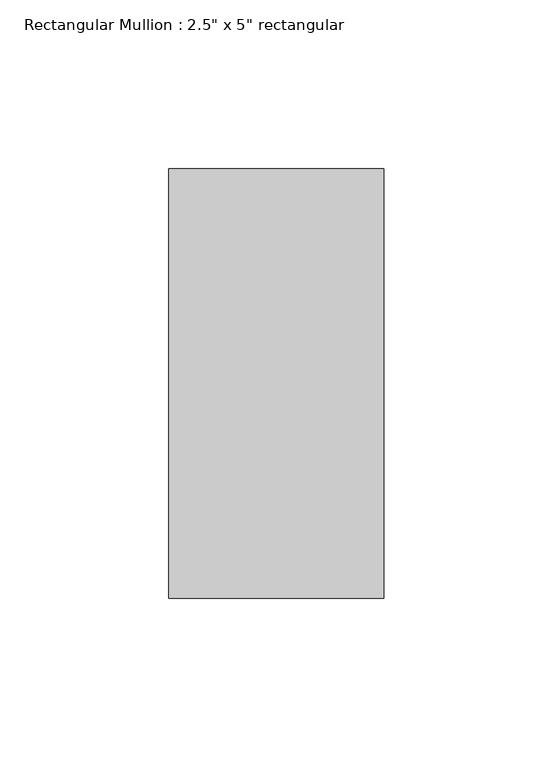
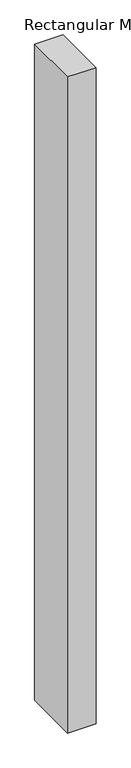
"""IFC4 building model written with IfcOpenShell, lengths in millimetres: member geometry."""

from ifc_helpers import new_model, si_unit, frame, origin, place, context, project, spatial, polyline, outline, extrude, source, transform, mapped, element, save


def member_8c7debe4(model_context):
    return source(origin(), model_context, "Body", "SweptSolid", [
        extrude(outline(polyline([(31.75, 63.5), (31.75, -63.5), (-31.75, -63.5), (-31.75, 63.5), (31.75, 63.5)])), frame((0.0, 0.0, -1550.242764), z_axis=(0.0, 0.0, 1.0), x_axis=(1.0, 0.0, 0.0)), (0.0, 0.0, 1.0), 1550.242764),
    ])


if __name__ == "__main__":
    model = new_model("IFC4")
    model_context = context("Model", 3, world=origin())
    ifc_project = project(units=[si_unit("LENGTHUNIT", "METRE", prefix="MILLI")], contexts=[model_context])
    site = spatial("IfcSite", under=ifc_project)
    building = spatial("IfcBuilding", under=site)
    placement = place(None, origin())
    member_shape = member_8c7debe4(model_context)
    element("IfcMember", 1, ObjectType="Rectangular Mullion : 2.5\" x 5\" rectangular", at=placement, inside=building, context=model_context, shape_type="MappedRepresentation", body=[
        mapped(member_shape, transform((0.0, 0.0, 0.0), x_axis=(1.0, 0.0, 0.0), y_axis=(0.0, 1.0, 0.0), z_axis=(0.0, 0.0, 1.0))),
    ])
    save(model, "model.ifc")

# Revit data of these elements
# Type "Rectangular Mullion : 2.5\" x 5\" rectangular"
#   built-in parameter 1007304 = 0.416667 (stored number, unit not read)
#   built-in parameter 1007301 = 0.104167 (stored number, unit not read)
#   built-in parameter 1007300 = 0.104167 (stored number, unit not read)
# Element 1 (IfcMember, "Rectangular Mullion : 2.5\" x 5\" rectangular")
#   Materials on its faces: "Aluminum"
# Materials
#   "Aluminum": class "Metal", colour RGB 247 247 247, transparency 0, Description = "Aluminum 6061", Cost = 0
